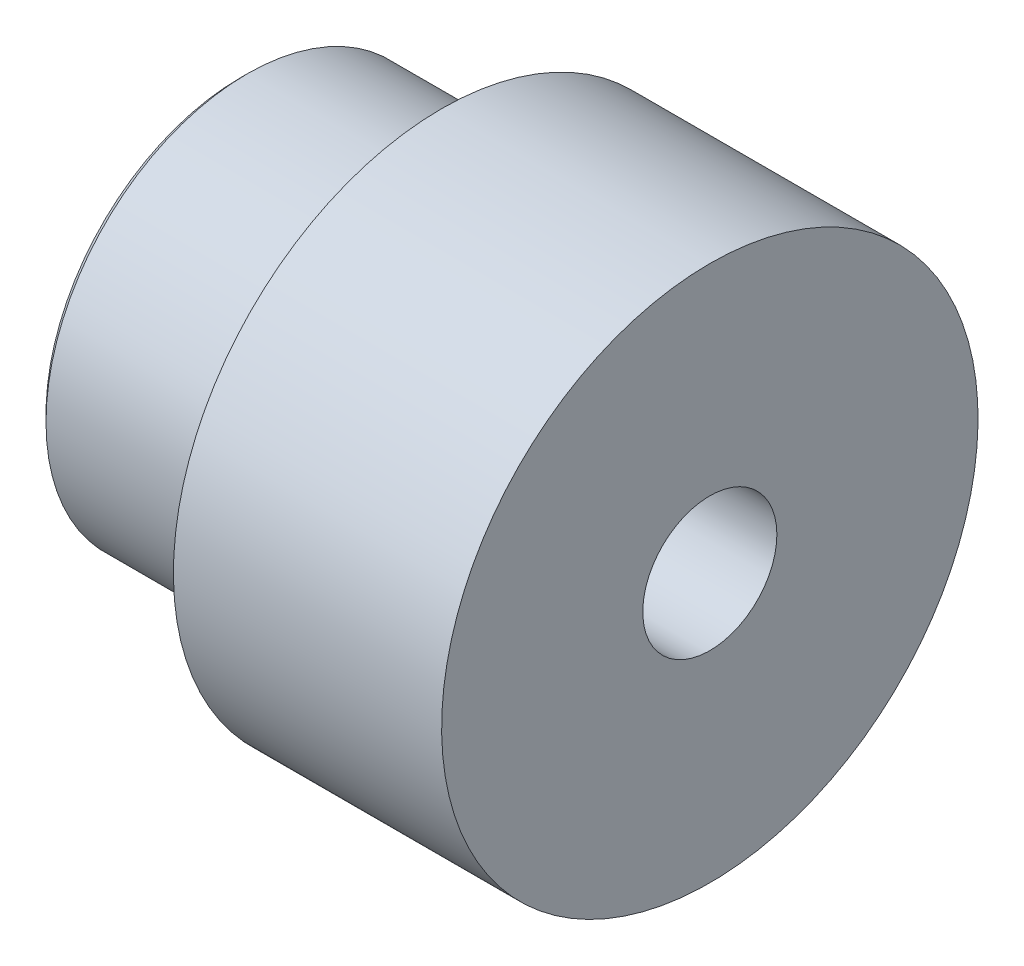
SolidWorks part; units mm, degrees
material "Plain Carbon Steel"
ref_plane "Front Plane" through (0, 0, 0) normal (0, 0, 1) x (1, 0, 0)
ref_plane "Top Plane" through (0, 0, 0) normal (0, 1, 0) x (1, 0, 0)
ref_plane "Right Plane" through (0, 0, 0) normal (1, 0, 0) x (0, 0, -1)
sketch "Turned Profile Sketch" plane through (0, 0, 0) normal (0, 0, 1) x (1, 0, 0)
  line L0 (0, 0) -> (0, 25.4)
  line L1 (0, 25.4) -> (-25.4, 25.4)
  line L2 (-25.4, 25.4) -> (-25.4, 19.05)
  line L3 (-0.941, 0) -> (0, 0)
  line L5 (-0.941, 0) -> (-44.45, 0)
  line L7 (-25.4, 19.05) -> (-44.45, 19.05)
  line L8 (-44.45, 0) -> (-44.45, 19.05)
  dimension "D1" = 44.45
  dimension "D2" = 19.05
  dimension "D3" = 25.4
  dimension "D4" = 19.05
  dimension "D5" = 0.941
revolve "Turned Body" add sketch "Turned Profile Sketch" angle 360 about L5
hole_wizard "Tapped Hole 1-4-20 x 0.5 Deep" positions "3DSketch3" profile "Sketch4" tap size "1/4-20" standard "ANSI Inch"
sketch3d "3DSketch3"
  point P0 (0, 0, 0)
  point P3 (0, 0, 0)
  point P5 (-44.45, 0, 0)
sketch "Sketch4" plane through (-44.45, 0, 0) normal (0, 1, 0) x (0, 0, 1)
  line L0 (0, 0) -> (0, 20.5838)
  line L1 (0, 20.5838) -> (2.5527, 19.05)
  line L2 (2.5527, 19.05) -> (2.5527, 12.7)
  line L3 (2.5527, 12.7) -> (3.175, 12.7)
  line L5 (3.175, 12.7) -> (3.175, 0.7305)
  line L6 (3.175, 0.7305) -> (3.81, 0)
  line L7 (3.81, 0) -> (0, 0)
  line L8 (-3.175, 0.7305) -> (-3.81, 0) construction
  line L10 (0, 20.5838) -> (-2.5527, 19.05) construction
  line L11 (0, -6.35) -> (0, 107.95) construction
  dimension "Tap Drill Dia." = 5.1054
  dimension "Tap Drill Depth" = 19.05
  dimension "Thread Major Dia." = 6.35
  dimension "Thread Depth" = 12.7
  dimension "Near C'Sink Dia." = 7.62
  dimension "Near C'Sink Angle" = 82
  dimension "Drill Angle" = 118
chamfer "Edge Chamfer 0.025in x 45deg" distance 0.635 angle 45 1 edges at (-44.45, 19.05, 0)
hole_wizard "Drilled Hole Ø0.5 x 0.75 Deep" positions "3DSketch4" profile "Sketch5" hole size "15/32" standard "ANSI Inch"
sketch3d "3DSketch4"
  point P0 (0, 0, 0)
sketch "Sketch5" plane through (0, 0, 0) normal (0, 1, 0) x (0, 0, -1)
  line L0 (0, 0) -> (0, 22.8655)
  line L1 (0, 22.8655) -> (6.35, 19.05)
  line L2 (6.35, 19.05) -> (6.35, 0)
  line L5 (6.35, 0) -> (0, 0)
  line L10 (0, 22.8655) -> (-6.35, 19.05) construction
  line L11 (0, -6.35) -> (0, 107.95) construction
  dimension "Hole Dia." = 12.7
  dimension "Hole Depth" = 19.05
  dimension "Drill Angle" = 118
